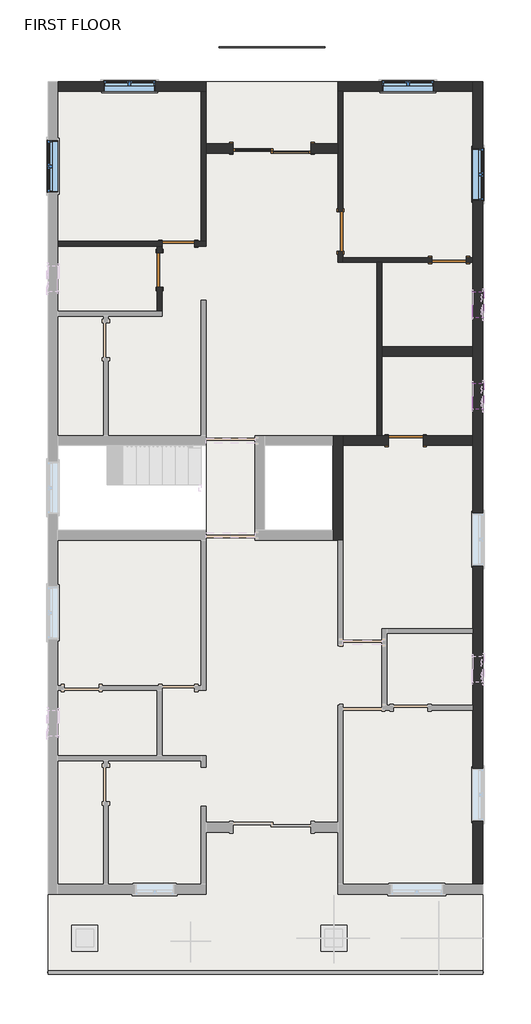
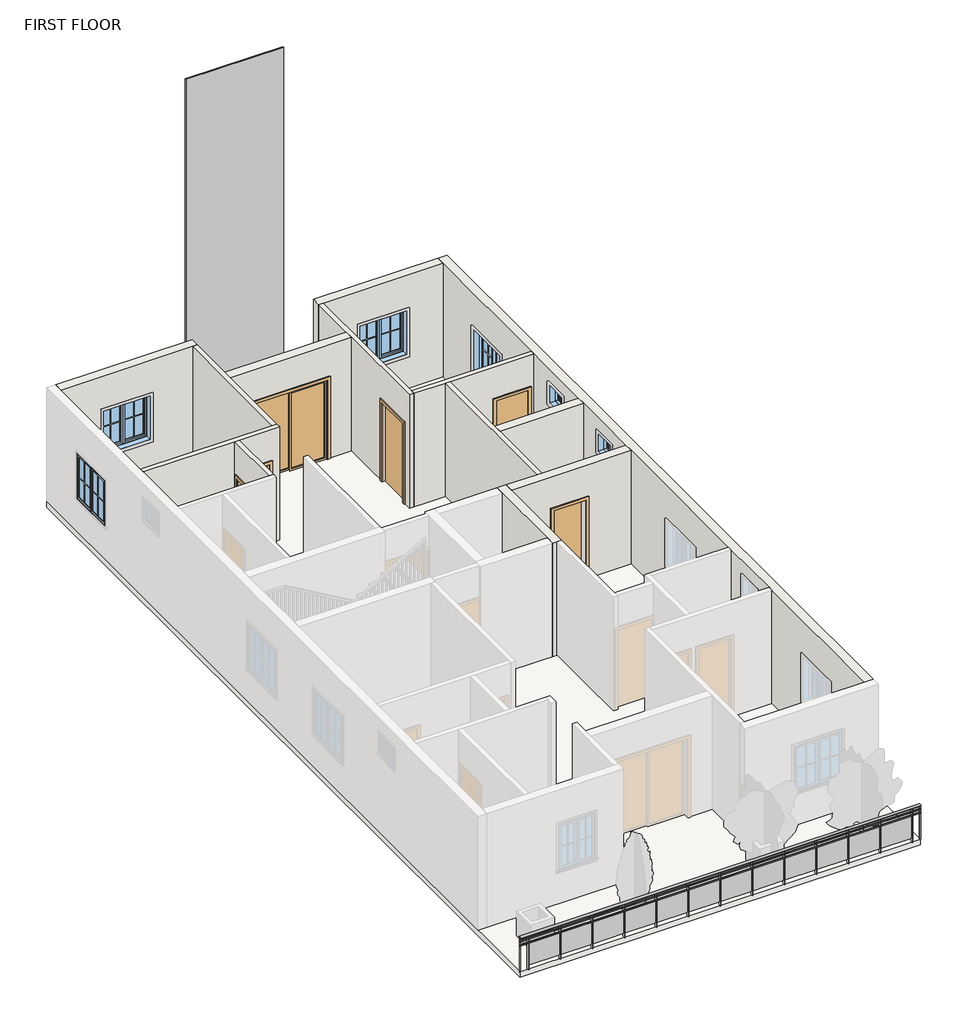
# One storey, part 2 of 4: 13 walls, 6 doors, 6 windows, 1 plate, 1 railing, 1 slab.
"""IFC4 building model written with IfcOpenShell, lengths in millimetres."""

from ifc_helpers import new_model, si_unit, point, frame, origin, place, context, project, spatial, polyline, ellipse_curve, trimmed, outline, extrude, faceted_brep, transform, mapped, element, save
from ifc_brep_helpers import plane_surface, extruded_surface, advanced_brep
from components import door_d4d75d1e, door_214872d5, door_d141acb4, door_38851409, door_7b345704, single_flush_3_x7_e5f9f3c4, system_panel_glazed_b4ce2d81, window_79894727, window_casement_double_4_x4_af3140d2

model = new_model("IFC4")

# Units and contexts
model_context = context("Model", 3, world=origin())
ifc_project = project(units=[si_unit("LENGTHUNIT", "METRE", prefix="MILLI")], contexts=[model_context])

# Site, building, storey
site = spatial("IfcSite", under=ifc_project)
building = spatial("IfcBuilding", under=site)
storey = spatial("IfcBuildingStorey", under=building, Name="FIRST FLOOR", Elevation=3200.4)

# Doors
placement = place(None, origin())
door_shape = door_d4d75d1e(model_context)
element("IfcDoor", 1, ObjectType="Door-Double-Sliding : 72\" x 84\"", at=placement, inside=storey, context=model_context, shape_type="MappedRepresentation", body=[
    mapped(door_shape, transform((-1119.4789041, 8623.7153263, 3200.4), x_axis=(-1.0, 0.0, 0.0), y_axis=(0.0, -1.0, 0.0), z_axis=(0.0, 0.0, 1.0))),
])
door_2_shape = door_214872d5(model_context)
element("IfcDoor", 2, ObjectType="Single-Flush : 2'6\"X7'", at=placement, inside=storey, context=model_context, shape_type="MappedRepresentation", body=[
    mapped(door_2_shape, transform((-3310.2289041, 6267.8653263, 3200.4), x_axis=(1.0, 0.0, 0.0), y_axis=(0.0, 1.0, 0.0), z_axis=(0.0, 0.0, 1.0))),
])
door_3_shape = door_d141acb4(model_context)
element("IfcDoor", 3, ObjectType="Single-Flush : 2'8\"X7'", at=placement, inside=storey, context=model_context, shape_type="MappedRepresentation", body=[
    mapped(door_3_shape, transform((-3748.3789041, 5651.9153263, 3200.4), x_axis=(0.0, 1.0, 0.0), y_axis=(-1.0, 0.0, 0.0), z_axis=(0.0, 0.0, 1.0))),
])
door_4_shape = door_38851409(model_context)
element("IfcDoor", 4, ObjectType="Single-Flush : 2'8\"X7'", at=placement, inside=storey, context=model_context, shape_type="MappedRepresentation", body=[
    mapped(door_4_shape, transform((3027.0710959, 5886.8653263, 3200.4), x_axis=(1.0, 0.0, 0.0), y_axis=(0.0, 1.0, 0.0), z_axis=(0.0, 0.0, 1.0))),
])
door_5_shape = door_7b345704(model_context)
element("IfcDoor", 5, ObjectType="Single-Flush : 2'8\"X7'", at=placement, inside=storey, context=model_context, shape_type="MappedRepresentation", body=[
    mapped(door_5_shape, transform((2011.0710959, 1664.1153263, 3200.4), x_axis=(-1.0, 0.0, 0.0), y_axis=(0.0, -1.0, 0.0), z_axis=(0.0, 0.0, 1.0))),
])
single_flush_3_x7_shape = single_flush_3_x7_e5f9f3c4(model_context)
element("IfcDoor", 6, ObjectType="Single-Flush : 3'X7'", at=placement, inside=storey, context=model_context, shape_type="MappedRepresentation", body=[
    mapped(single_flush_3_x7_shape, transform((480.7210959, 6553.6153263, 3200.4), x_axis=(0.0, -1.0, 0.0), y_axis=(1.0, 0.0, 0.0), z_axis=(0.0, 0.0, 1.0))),
])

# Plate
system_panel_glazed_shape = system_panel_glazed_b4ce2d81(model_context)
element("IfcPlate", 7, ObjectType="System Panel : Glazed", at=placement, inside=storey, context=model_context, shape_type="MappedRepresentation", body=[
    mapped(system_panel_glazed_shape, transform((-1119.4789041, 10833.5153263, 3200.4), x_axis=(1.0, 0.0, 0.0), y_axis=(0.0, 1.0, 0.0), z_axis=(0.0, 0.0, 1.0))),
])

# Railing
element("IfcRailing", 8, ObjectType="Glass Panel - Bottom Fill", at=placement, inside=storey, context=model_context, shape_type="SolidModel", body=[
    advanced_brep(
    [(-6358.2289041, -10731.0846737, 4114.8), (-6358.2289041, -10807.2846737, 4114.8), (3814.4710959, -10731.0846737, 4114.8), (3814.4710959, -10807.2846737, 4114.8)],
    [
        (0, 1, ellipse_curve(frame((-6358.2289041, -10769.1846737, 4114.8), z_axis=(-1.0, 0.0, 0.0), x_axis=(0.0, -1.0, 0.0)), 38.1, 28.575)),
        (1, 0, ellipse_curve(frame((-6358.2289041, -10769.1846737, 4114.8), z_axis=(-1.0, 0.0, 0.0), x_axis=(0.0, -1.0, 0.0)), 38.1, 28.575)),
        (2, 3, ellipse_curve(frame((3814.4710959, -10769.1846737, 4114.8), z_axis=(1.0, 0.0, 0.0), x_axis=(0.0, -1.0, 0.0)), 38.1, 28.575)),
        (3, 2, ellipse_curve(frame((3814.4710959, -10769.1846737, 4114.8), z_axis=(1.0, 0.0, 0.0), x_axis=(0.0, -1.0, 0.0)), 38.1, 28.575)),
        (0, 2),
        (3, 1),
    ],
    [
        plane_surface(frame((-6358.2289041, -10769.1846737, 4114.8), z_axis=(-1.0, 0.0, 0.0), x_axis=(0.0, 1.0, 0.0))),
        plane_surface(frame((3814.4710959, -10769.1846737, 4114.8), z_axis=(1.0, 0.0, 0.0), x_axis=(0.0, 1.0, 0.0))),
        extruded_surface(trimmed(ellipse_curve(frame((3814.4710959, -10769.1846737, 4114.8), z_axis=(-1.0, 0.0, 0.0), x_axis=(0.0, -1.0, 0.0)), 38.1, 28.575), [point((3814.4710959, -10731.0846737, 4114.8))], [point((3814.4710959, -10807.2846737, 4114.8))], True, "CARTESIAN"), (-10172.7, 0.0, 0.0), 10172.7),
        extruded_surface(trimmed(ellipse_curve(frame((3814.4710959, -10769.1846737, 4114.8), z_axis=(-1.0, 0.0, 0.0), x_axis=(0.0, -1.0, 0.0)), 38.1, 28.575), [point((3814.4710959, -10807.2846737, 4114.8))], [point((3814.4710959, -10731.0846737, 4114.8))], True, "CARTESIAN"), (-10172.7, 0.0, 0.0), 10172.7),
    ],
    [
        (0, [[1, 2]]),
        (1, [[3, 4]]),
        (2, [[-1, 5, -4, 6]]),
        (3, [[-2, -6, -3, -5]]),
    ],
),
    extrude(outline(polyline([(-6358.2289041, -10781.8846737), (-6358.2289041, -10756.4846737), (3814.4710959, -10756.4846737), (3814.4710959, -10781.8846737), (-6358.2289041, -10781.8846737)])), frame((0.0, 0.0, 4000.5), z_axis=(0.0, 0.0, 1.0), x_axis=(1.0, 0.0, 0.0)), (0.0, 0.0, 1.0), 25.4),
    extrude(outline(polyline([(-6358.2289041, -10781.8846737), (-6358.2289041, -10756.4846737), (3814.4710959, -10756.4846737), (3814.4710959, -10781.8846737), (-6358.2289041, -10781.8846737)])), frame((0.0, 0.0, 3898.9), z_axis=(0.0, 0.0, 1.0), x_axis=(1.0, 0.0, 0.0)), (0.0, 0.0, 1.0), 25.4),
    extrude(outline(polyline([(3598.5710959, -10794.5846737), (3598.5710959, -10743.7846737), (3611.2710959, -10743.7846737), (3611.2710959, -10794.5846737), (3598.5710959, -10794.5846737)])), frame((0.0, 0.0, 3200.4), z_axis=(0.0, 0.0, 1.0), x_axis=(1.0, 0.0, 0.0)), (0.0, 0.0, 1.0), 885.825),
    extrude(outline(polyline([(2792.1210959, -10762.6495167), (3604.9210959, -10762.6495167), (3604.9210959, -10768.9995167), (2792.1210959, -10768.9995167), (2792.1210959, -10762.6495167)])), frame((0.0, 0.0, 3302.0), z_axis=(0.0, 0.0, 1.0), x_axis=(1.0, 0.0, 0.0)), (0.0, 0.0, 1.0), 596.9),
    extrude(outline(polyline([(2785.7710959, -10794.5846737), (2785.7710959, -10743.7846737), (2798.4710959, -10743.7846737), (2798.4710959, -10794.5846737), (2785.7710959, -10794.5846737)])), frame((0.0, 0.0, 3200.4), z_axis=(0.0, 0.0, 1.0), x_axis=(1.0, 0.0, 0.0)), (0.0, 0.0, 1.0), 885.825),
    extrude(outline(polyline([(1979.3210959, -10762.6495167), (2792.1210959, -10762.6495167), (2792.1210959, -10768.9995167), (1979.3210959, -10768.9995167), (1979.3210959, -10762.6495167)])), frame((0.0, 0.0, 3302.0), z_axis=(0.0, 0.0, 1.0), x_axis=(1.0, 0.0, 0.0)), (0.0, 0.0, 1.0), 596.9),
    extrude(outline(polyline([(1972.9710959, -10794.5846737), (1972.9710959, -10743.7846737), (1985.6710959, -10743.7846737), (1985.6710959, -10794.5846737), (1972.9710959, -10794.5846737)])), frame((0.0, 0.0, 3200.4), z_axis=(0.0, 0.0, 1.0), x_axis=(1.0, 0.0, 0.0)), (0.0, 0.0, 1.0), 885.825),
    extrude(outline(polyline([(1166.5210959, -10762.6495167), (1979.3210959, -10762.6495167), (1979.3210959, -10768.9995167), (1166.5210959, -10768.9995167), (1166.5210959, -10762.6495167)])), frame((0.0, 0.0, 3302.0), z_axis=(0.0, 0.0, 1.0), x_axis=(1.0, 0.0, 0.0)), (0.0, 0.0, 1.0), 596.9),
    extrude(outline(polyline([(1160.1710959, -10794.5846737), (1160.1710959, -10743.7846737), (1172.8710959, -10743.7846737), (1172.8710959, -10794.5846737), (1160.1710959, -10794.5846737)])), frame((0.0, 0.0, 3200.4), z_axis=(0.0, 0.0, 1.0), x_axis=(1.0, 0.0, 0.0)), (0.0, 0.0, 1.0), 885.825),
    extrude(outline(polyline([(353.7210959, -10762.6495167), (1166.5210959, -10762.6495167), (1166.5210959, -10768.9995167), (353.7210959, -10768.9995167), (353.7210959, -10762.6495167)])), frame((0.0, 0.0, 3302.0), z_axis=(0.0, 0.0, 1.0), x_axis=(1.0, 0.0, 0.0)), (0.0, 0.0, 1.0), 596.9),
    extrude(outline(polyline([(347.3710959, -10794.5846737), (347.3710959, -10743.7846737), (360.0710959, -10743.7846737), (360.0710959, -10794.5846737), (347.3710959, -10794.5846737)])), frame((0.0, 0.0, 3200.4), z_axis=(0.0, 0.0, 1.0), x_axis=(1.0, 0.0, 0.0)), (0.0, 0.0, 1.0), 885.825),
    extrude(outline(polyline([(-459.0789041, -10762.6495167), (353.7210959, -10762.6495167), (353.7210959, -10768.9995167), (-459.0789041, -10768.9995167), (-459.0789041, -10762.6495167)])), frame((0.0, 0.0, 3302.0), z_axis=(0.0, 0.0, 1.0), x_axis=(1.0, 0.0, 0.0)), (0.0, 0.0, 1.0), 596.9),
    extrude(outline(polyline([(-465.4289041, -10794.5846737), (-465.4289041, -10743.7846737), (-452.7289041, -10743.7846737), (-452.7289041, -10794.5846737), (-465.4289041, -10794.5846737)])), frame((0.0, 0.0, 3200.4), z_axis=(0.0, 0.0, 1.0), x_axis=(1.0, 0.0, 0.0)), (0.0, 0.0, 1.0), 885.825),
    extrude(outline(polyline([(-1271.8789041, -10762.6495167), (-459.0789041, -10762.6495167), (-459.0789041, -10768.9995167), (-1271.8789041, -10768.9995167), (-1271.8789041, -10762.6495167)])), frame((0.0, 0.0, 3302.0), z_axis=(0.0, 0.0, 1.0), x_axis=(1.0, 0.0, 0.0)), (0.0, 0.0, 1.0), 596.9),
    extrude(outline(polyline([(-1278.2289041, -10794.5846737), (-1278.2289041, -10743.7846737), (-1265.5289041, -10743.7846737), (-1265.5289041, -10794.5846737), (-1278.2289041, -10794.5846737)])), frame((0.0, 0.0, 3200.4), z_axis=(0.0, 0.0, 1.0), x_axis=(1.0, 0.0, 0.0)), (0.0, 0.0, 1.0), 885.825),
    extrude(outline(polyline([(-2084.6789041, -10762.6495167), (-1271.8789041, -10762.6495167), (-1271.8789041, -10768.9995167), (-2084.6789041, -10768.9995167), (-2084.6789041, -10762.6495167)])), frame((0.0, 0.0, 3302.0), z_axis=(0.0, 0.0, 1.0), x_axis=(1.0, 0.0, 0.0)), (0.0, 0.0, 1.0), 596.9),
    extrude(outline(polyline([(-2091.0289041, -10794.5846737), (-2091.0289041, -10743.7846737), (-2078.3289041, -10743.7846737), (-2078.3289041, -10794.5846737), (-2091.0289041, -10794.5846737)])), frame((0.0, 0.0, 3200.4), z_axis=(0.0, 0.0, 1.0), x_axis=(1.0, 0.0, 0.0)), (0.0, 0.0, 1.0), 885.825),
    extrude(outline(polyline([(-2897.4789041, -10762.6495167), (-2084.6789041, -10762.6495167), (-2084.6789041, -10768.9995167), (-2897.4789041, -10768.9995167), (-2897.4789041, -10762.6495167)])), frame((0.0, 0.0, 3302.0), z_axis=(0.0, 0.0, 1.0), x_axis=(1.0, 0.0, 0.0)), (0.0, 0.0, 1.0), 596.9),
    extrude(outline(polyline([(-2903.8289041, -10794.5846737), (-2903.8289041, -10743.7846737), (-2891.1289041, -10743.7846737), (-2891.1289041, -10794.5846737), (-2903.8289041, -10794.5846737)])), frame((0.0, 0.0, 3200.4), z_axis=(0.0, 0.0, 1.0), x_axis=(1.0, 0.0, 0.0)), (0.0, 0.0, 1.0), 885.825),
    extrude(outline(polyline([(-3710.2789041, -10762.6495167), (-2897.4789041, -10762.6495167), (-2897.4789041, -10768.9995167), (-3710.2789041, -10768.9995167), (-3710.2789041, -10762.6495167)])), frame((0.0, 0.0, 3302.0), z_axis=(0.0, 0.0, 1.0), x_axis=(1.0, 0.0, 0.0)), (0.0, 0.0, 1.0), 596.9),
    extrude(outline(polyline([(-3716.6289041, -10794.5846737), (-3716.6289041, -10743.7846737), (-3703.9289041, -10743.7846737), (-3703.9289041, -10794.5846737), (-3716.6289041, -10794.5846737)])), frame((0.0, 0.0, 3200.4), z_axis=(0.0, 0.0, 1.0), x_axis=(1.0, 0.0, 0.0)), (0.0, 0.0, 1.0), 885.825),
    extrude(outline(polyline([(-4523.0789041, -10762.6495167), (-3710.2789041, -10762.6495167), (-3710.2789041, -10768.9995167), (-4523.0789041, -10768.9995167), (-4523.0789041, -10762.6495167)])), frame((0.0, 0.0, 3302.0), z_axis=(0.0, 0.0, 1.0), x_axis=(1.0, 0.0, 0.0)), (0.0, 0.0, 1.0), 596.9),
    extrude(outline(polyline([(-4529.4289041, -10794.5846737), (-4529.4289041, -10743.7846737), (-4516.7289041, -10743.7846737), (-4516.7289041, -10794.5846737), (-4529.4289041, -10794.5846737)])), frame((0.0, 0.0, 3200.4), z_axis=(0.0, 0.0, 1.0), x_axis=(1.0, 0.0, 0.0)), (0.0, 0.0, 1.0), 885.825),
    extrude(outline(polyline([(-5335.8789041, -10762.6495167), (-4523.0789041, -10762.6495167), (-4523.0789041, -10768.9995167), (-5335.8789041, -10768.9995167), (-5335.8789041, -10762.6495167)])), frame((0.0, 0.0, 3302.0), z_axis=(0.0, 0.0, 1.0), x_axis=(1.0, 0.0, 0.0)), (0.0, 0.0, 1.0), 596.9),
    extrude(outline(polyline([(-5342.2289041, -10794.5846737), (-5342.2289041, -10743.7846737), (-5329.5289041, -10743.7846737), (-5329.5289041, -10794.5846737), (-5342.2289041, -10794.5846737)])), frame((0.0, 0.0, 3200.4), z_axis=(0.0, 0.0, 1.0), x_axis=(1.0, 0.0, 0.0)), (0.0, 0.0, 1.0), 885.825),
    extrude(outline(polyline([(-6148.6789041, -10762.6495167), (-5335.8789041, -10762.6495167), (-5335.8789041, -10768.9995167), (-6148.6789041, -10768.9995167), (-6148.6789041, -10762.6495167)])), frame((0.0, 0.0, 3302.0), z_axis=(0.0, 0.0, 1.0), x_axis=(1.0, 0.0, 0.0)), (0.0, 0.0, 1.0), 596.9),
    extrude(outline(polyline([(-6155.0289041, -10794.5846737), (-6155.0289041, -10743.7846737), (-6142.3289041, -10743.7846737), (-6142.3289041, -10794.5846737), (-6155.0289041, -10794.5846737)])), frame((0.0, 0.0, 3200.4), z_axis=(0.0, 0.0, 1.0), x_axis=(1.0, 0.0, 0.0)), (0.0, 0.0, 1.0), 885.825),
    extrude(outline(polyline([(3801.7710959, -10778.7096737), (3801.7710959, -10759.6596737), (3820.8210959, -10759.6596737), (3820.8210959, -10778.7096737), (3801.7710959, -10778.7096737)])), frame((0.0, 0.0, 3200.4), z_axis=(0.0, 0.0, 1.0), x_axis=(1.0, 0.0, 0.0)), (0.0, 0.0, 1.0), 885.825),
    extrude(outline(polyline([(-6364.5789041, -10778.7096737), (-6364.5789041, -10759.6596737), (-6345.5289041, -10759.6596737), (-6345.5289041, -10778.7096737), (-6364.5789041, -10778.7096737)])), frame((0.0, 0.0, 3200.4), z_axis=(0.0, 0.0, 1.0), x_axis=(1.0, 0.0, 0.0)), (0.0, 0.0, 1.0), 885.825),
])

# Slab
element("IfcSlab", 9, ObjectType="6\"", at=placement, inside=storey, context=model_context, shape_type="SweptSolid", body=[
    extrude(outline(polyline([(3814.4710959, 10058.8153263), (3814.4710959, -10769.1846737), (-6358.2289041, -10769.1846737), (-6358.2289041, 10058.8153263), (3814.4710959, 10058.8153263)]), holes=[polyline([(-2662.5289041, 1549.8153263), (-6129.6289041, 1549.8153263), (-6129.6289041, -431.3846737), (-2662.5289041, -431.3846737), (-2662.5289041, 1549.8153263)]), polyline([(537.8710959, 1778.4153263), (-1519.5289041, 1778.4153263), (-1519.5289041, -659.9846737), (537.8710959, -659.9846737), (537.8710959, 1778.4153263)])]), frame((0.0, 0.0, 3048.0), z_axis=(0.0, 0.0, 1.0), x_axis=(1.0, 0.0, 0.0)), (0.0, 0.0, 1.0), 152.4),
])

# Walls
element("IfcWall", 10, ObjectType="4.5\"", at=placement, inside=storey, context=model_context, shape_type="SweptSolid", body=[
    extrude(outline(polyline([(6210.7153263, 3200.4), (6058.3153263, 3200.4), (6058.3153263, 5334.0), (5245.5153263, 5334.0), (5245.5153263, 3200.4), (4686.7153263, 3200.4), (4686.7153263, 6248.4), (6210.7153263, 6248.4), (6210.7153263, 3200.4)])), frame((-3805.5289041, 0.0, 0.0), z_axis=(1.0, 0.0, 0.0), x_axis=(0.0, 1.0, 0.0)), (0.0, 0.0, 1.0), 114.3),
])
element("IfcWall", 11, ObjectType="4.5\"", at=placement, inside=storey, context=model_context, shape_type="Brep", body=[
    faceted_brep([(-2929.2289041, 6210.7153263, 5334.0), (-2929.2289041, 6210.7153263, 3200.4), (-2662.5289041, 6210.7153263, 3200.4), (-2662.5289041, 6210.7153263, 6248.4), (-3691.2289041, 6210.7153263, 6248.4), (-3805.5289041, 6210.7153263, 6248.4), (-6129.6289041, 6210.7153263, 6248.4), (-6129.6289041, 6210.7153263, 3200.4), (-3805.5289041, 6210.7153263, 3200.4), (-3691.2289041, 6210.7153263, 3200.4), (-3691.2289041, 6210.7153263, 5334.0), (-2662.5289041, 6325.0153263, 3200.4), (-2776.8289041, 6325.0153263, 3200.4), (-2929.2289041, 6325.0153263, 3200.4), (-2929.2289041, 6325.0153263, 5334.0), (-3691.2289041, 6325.0153263, 5334.0), (-3691.2289041, 6325.0153263, 3200.4), (-6129.6289041, 6325.0153263, 3200.4), (-6129.6289041, 6325.0153263, 6248.4), (-2776.8289041, 6325.0153263, 6248.4), (-2662.5289041, 6325.0153263, 6248.4)], [[[0, 1, 2, 3, 4, 5, 6, 7, 8, 9, 10]], [[11, 12, 13, 14, 15, 16, 17, 18, 19, 20]], [[2, 1, 13, 12, 11]], [[9, 8, 7, 17, 16]], [[6, 5, 4, 3, 20, 19, 18]], [[7, 6, 18, 17]], [[3, 2, 11, 20]], [[14, 13, 1, 0]], [[15, 14, 0, 10]], [[16, 15, 10, 9]]]),
])
element("IfcWall", 12, ObjectType="4.5\"", at=placement, inside=storey, context=model_context, shape_type="Brep", body=[
    faceted_brep([(-2662.5289041, 6325.0153263, 3200.4), (-2662.5289041, 8382.4153263, 3200.4), (-2662.5289041, 8611.0153263, 3200.4), (-2662.5289041, 9830.2153263, 3200.4), (-2662.5289041, 9830.2153263, 6248.4), (-2662.5289041, 8611.0153263, 6248.4), (-2662.5289041, 8382.4153263, 6248.4), (-2662.5289041, 6325.0153263, 6248.4), (-2776.8289041, 6325.0153263, 3200.4), (-2776.8289041, 6325.0153263, 6248.4), (-2776.8289041, 9830.2153263, 6248.4), (-2776.8289041, 9830.2153263, 3200.4)], [[[0, 1, 2, 3, 4, 5, 6, 7]], [[8, 9, 10, 11]], [[3, 2, 1, 0, 8, 11]], [[7, 6, 5, 4, 10, 9]], [[0, 7, 9, 8]], [[4, 3, 11, 10]]]),
])
element("IfcWall", 13, ObjectType="4.5\"", at=placement, inside=storey, context=model_context, shape_type="Brep", body=[
    faceted_brep([(423.5710959, 6096.4153263, 5334.0), (423.5710959, 6096.4153263, 3200.4), (423.5710959, 5829.7153263, 3200.4), (423.5710959, 5829.7153263, 6248.4), (423.5710959, 8382.4153263, 6248.4), (423.5710959, 8611.0153263, 6248.4), (423.5710959, 9830.2153263, 6248.4), (423.5710959, 9830.2153263, 3200.4), (423.5710959, 8611.0153263, 3200.4), (423.5710959, 8382.4153263, 3200.4), (423.5710959, 7010.8153263, 3200.4), (423.5710959, 7010.8153263, 5334.0), (537.8710959, 5829.7153263, 3200.4), (537.8710959, 5944.0153263, 3200.4), (537.8710959, 6096.4153263, 3200.4), (537.8710959, 6096.4153263, 5334.0), (537.8710959, 7010.8153263, 5334.0), (537.8710959, 7010.8153263, 3200.4), (537.8710959, 9830.2153263, 3200.4), (537.8710959, 9830.2153263, 6248.4), (537.8710959, 5944.0153263, 6248.4), (537.8710959, 5829.7153263, 6248.4)], [[[0, 1, 2, 3, 4, 5, 6, 7, 8, 9, 10, 11]], [[12, 13, 14, 15, 16, 17, 18, 19, 20, 21]], [[2, 1, 14, 13, 12]], [[10, 9, 8, 7, 18, 17]], [[6, 5, 4, 3, 21, 20, 19]], [[7, 6, 19, 18]], [[3, 2, 12, 21]], [[15, 14, 1, 0]], [[16, 15, 0, 11]], [[17, 16, 11, 10]]]),
])
element("IfcWall", 14, ObjectType="4.5\"", at=placement, inside=storey, context=model_context, shape_type="Brep", body=[
    faceted_brep([(3433.4710959, 5829.7153263, 5334.0), (3433.4710959, 5829.7153263, 3200.4), (3585.8710959, 5829.7153263, 3200.4), (3585.8710959, 5829.7153263, 6248.4), (1452.2710959, 5829.7153263, 6248.4), (1337.9710959, 5829.7153263, 6248.4), (537.8710959, 5829.7153263, 6248.4), (537.8710959, 5829.7153263, 3200.4), (1337.9710959, 5829.7153263, 3200.4), (1452.2710959, 5829.7153263, 3200.4), (2620.6710959, 5829.7153263, 3200.4), (2620.6710959, 5829.7153263, 5334.0), (3585.8710959, 5944.0153263, 3200.4), (3433.4710959, 5944.0153263, 3200.4), (3433.4710959, 5944.0153263, 5334.0), (2620.6710959, 5944.0153263, 5334.0), (2620.6710959, 5944.0153263, 3200.4), (537.8710959, 5944.0153263, 3200.4), (537.8710959, 5944.0153263, 6248.4), (3585.8710959, 5944.0153263, 6248.4)], [[[0, 1, 2, 3, 4, 5, 6, 7, 8, 9, 10, 11]], [[12, 13, 14, 15, 16, 17, 18, 19]], [[2, 1, 13, 12]], [[10, 9, 8, 7, 17, 16]], [[6, 5, 4, 3, 19, 18]], [[7, 6, 18, 17]], [[3, 2, 12, 19]], [[14, 13, 1, 0]], [[15, 14, 0, 11]], [[16, 15, 11, 10]]]),
])
element("IfcWall", 15, ObjectType="4.5\"", at=placement, inside=storey, context=model_context, shape_type="Brep", body=[
    faceted_brep([(1337.9710959, 5829.7153263, 3200.4), (1337.9710959, 1778.4153263, 3200.4), (1337.9710959, 1778.4153263, 6248.4), (1337.9710959, 5829.7153263, 6248.4), (1452.2710959, 5829.7153263, 3200.4), (1452.2710959, 5829.7153263, 6248.4), (1452.2710959, 3861.2153263, 6248.4), (1452.2710959, 3632.6153263, 6248.4), (1452.2710959, 1778.4153263, 6248.4), (1452.2710959, 1778.4153263, 3200.4), (1452.2710959, 3632.6153263, 3200.4), (1452.2710959, 3861.2153263, 3200.4)], [[[0, 1, 2, 3]], [[4, 5, 6, 7, 8, 9, 10, 11]], [[1, 0, 4, 11, 10, 9]], [[3, 2, 8, 7, 6, 5]], [[2, 1, 9, 8]], [[0, 3, 5, 4]]]),
])
element("IfcWall", 16, ObjectType="9\"", at=placement, inside=storey, context=model_context, shape_type="Brep", body=[
    faceted_brep([(3814.4710959, -8711.7846737, 3200.4), (3814.4710959, 10058.8153263, 3200.4), (3814.4710959, 10058.8153263, 6248.4), (3814.4710959, -8711.7846737, 6248.4), (3814.4710959, -7225.8846737, 5334.0), (3814.4710959, -6006.6846737, 5334.0), (3814.4710959, -6006.6846737, 4114.8), (3814.4710959, -7225.8846737, 4114.8), (3814.4710959, -1256.8846737, 5334.0), (3814.4710959, -37.6846737, 5334.0), (3814.4710959, -37.6846737, 4114.8), (3814.4710959, -1256.8846737, 4114.8), (3814.4710959, 7277.5153263, 5334.0), (3814.4710959, 8496.7153263, 5334.0), (3814.4710959, 8496.7153263, 4114.8), (3814.4710959, 7277.5153263, 4114.8), (3814.4710959, -3987.3846737, 5867.4), (3814.4710959, -3377.7846737, 5867.4), (3814.4710959, -3377.7846737, 5334.0), (3814.4710959, -3987.3846737, 5334.0), (3814.4710959, 2400.7153263, 5867.4), (3814.4710959, 3010.3153263, 5867.4), (3814.4710959, 3010.3153263, 5334.0), (3814.4710959, 2400.7153263, 5334.0), (3814.4710959, 4540.6653263, 5867.4), (3814.4710959, 5150.2653263, 5867.4), (3814.4710959, 5150.2653263, 5334.0), (3814.4710959, 4540.6653263, 5334.0), (3585.8710959, -8711.7846737, 3200.4), (3585.8710959, -8711.7846737, 6248.4), (3585.8710959, -4635.0846737, 6248.4), (3585.8710959, -4520.7846737, 6248.4), (3585.8710959, -2844.3846737, 6248.4), (3585.8710959, -2730.0846737, 6248.4), (3585.8710959, 1549.8153263, 6248.4), (3585.8710959, 1778.4153263, 6248.4), (3585.8710959, 3632.6153263, 6248.4), (3585.8710959, 3861.2153263, 6248.4), (3585.8710959, 5829.7153263, 6248.4), (3585.8710959, 5944.0153263, 6248.4), (3585.8710959, 9830.2153263, 6248.4), (3585.8710959, 10058.8153263, 6248.4), (3585.8710959, 10058.8153263, 3200.4), (3585.8710959, 9830.2153263, 3200.4), (3585.8710959, 5944.0153263, 3200.4), (3585.8710959, 5829.7153263, 3200.4), (3585.8710959, 3861.2153263, 3200.4), (3585.8710959, 3632.6153263, 3200.4), (3585.8710959, 1778.4153263, 3200.4), (3585.8710959, 1549.8153263, 3200.4), (3585.8710959, -2730.0846737, 3200.4), (3585.8710959, -2844.3846737, 3200.4), (3585.8710959, -4520.7846737, 3200.4), (3585.8710959, -4635.0846737, 3200.4), (3585.8710959, -7225.8846737, 5334.0), (3585.8710959, -7225.8846737, 4114.8), (3585.8710959, -6006.6846737, 4114.8), (3585.8710959, -6006.6846737, 5334.0), (3585.8710959, -1256.8846737, 5334.0), (3585.8710959, -1256.8846737, 4114.8), (3585.8710959, -37.6846737, 4114.8), (3585.8710959, -37.6846737, 5334.0), (3585.8710959, 7277.5153263, 5334.0), (3585.8710959, 7277.5153263, 4114.8), (3585.8710959, 8496.7153263, 4114.8), (3585.8710959, 8496.7153263, 5334.0), (3585.8710959, -3987.3846737, 5867.4), (3585.8710959, -3987.3846737, 5334.0), (3585.8710959, -3377.7846737, 5334.0), (3585.8710959, -3377.7846737, 5867.4), (3585.8710959, 2400.7153263, 5867.4), (3585.8710959, 2400.7153263, 5334.0), (3585.8710959, 3010.3153263, 5334.0), (3585.8710959, 3010.3153263, 5867.4), (3585.8710959, 4540.6653263, 5867.4), (3585.8710959, 4540.6653263, 5334.0), (3585.8710959, 5150.2653263, 5334.0), (3585.8710959, 5150.2653263, 5867.4)], [[[0, 1, 2, 3], [4, 5, 6, 7], [8, 9, 10, 11], [12, 13, 14, 15], [16, 17, 18, 19], [20, 21, 22, 23], [24, 25, 26, 27]], [[28, 29, 30, 31, 32, 33, 34, 35, 36, 37, 38, 39, 40, 41, 42, 43, 44, 45, 46, 47, 48, 49, 50, 51, 52, 53], [54, 55, 56, 57], [58, 59, 60, 61], [62, 63, 64, 65], [66, 67, 68, 69], [70, 71, 72, 73], [74, 75, 76, 77]], [[1, 0, 28, 53, 52, 51, 50, 49, 48, 47, 46, 45, 44, 43, 42]], [[3, 2, 41, 40, 39, 38, 37, 36, 35, 34, 33, 32, 31, 30, 29]], [[0, 3, 29, 28]], [[2, 1, 42, 41]], [[55, 54, 4, 7]], [[56, 55, 7, 6]], [[57, 56, 6, 5]], [[54, 57, 5, 4]], [[59, 58, 8, 11]], [[60, 59, 11, 10]], [[61, 60, 10, 9]], [[58, 61, 9, 8]], [[63, 62, 12, 15]], [[64, 63, 15, 14]], [[65, 64, 14, 13]], [[62, 65, 13, 12]], [[67, 66, 16, 19]], [[68, 67, 19, 18]], [[69, 68, 18, 17]], [[66, 69, 17, 16]], [[71, 70, 20, 23]], [[72, 71, 23, 22]], [[73, 72, 22, 21]], [[70, 73, 21, 20]], [[75, 74, 24, 27]], [[76, 75, 27, 26]], [[77, 76, 26, 25]], [[74, 77, 25, 24]]]),
])
element("IfcWall", 17, ObjectType="9\"", at=placement, inside=storey, context=model_context, shape_type="Brep", body=[
    faceted_brep([(3585.8710959, 10058.8153263, 3200.4), (423.5710959, 10058.8153263, 3200.4), (423.5710959, 10058.8153263, 6248.4), (3585.8710959, 10058.8153263, 6248.4), (2671.4710959, 10058.8153263, 5334.0), (1452.2710959, 10058.8153263, 5334.0), (1452.2710959, 10058.8153263, 4114.8), (2671.4710959, 10058.8153263, 4114.8), (3585.8710959, 9830.2153263, 3200.4), (3585.8710959, 9830.2153263, 6248.4), (537.8710959, 9830.2153263, 6248.4), (423.5710959, 9830.2153263, 6248.4), (423.5710959, 9830.2153263, 3200.4), (537.8710959, 9830.2153263, 3200.4), (2671.4710959, 9830.2153263, 5334.0), (2671.4710959, 9830.2153263, 4114.8), (1452.2710959, 9830.2153263, 4114.8), (1452.2710959, 9830.2153263, 5334.0)], [[[0, 1, 2, 3], [4, 5, 6, 7]], [[8, 9, 10, 11, 12, 13], [14, 15, 16, 17]], [[1, 0, 8, 13, 12]], [[3, 2, 11, 10, 9]], [[0, 3, 9, 8]], [[2, 1, 12, 11]], [[15, 14, 4, 7]], [[16, 15, 7, 6]], [[17, 16, 6, 5]], [[14, 17, 5, 4]]]),
])
element("IfcWall", 18, ObjectType="9\"", at=placement, inside=storey, context=model_context, shape_type="Brep", body=[
    faceted_brep([(-2662.5289041, 10058.8153263, 3200.4), (-6129.6289041, 10058.8153263, 3200.4), (-6129.6289041, 10058.8153263, 6248.4), (-2662.5289041, 10058.8153263, 6248.4), (-3843.6289041, 10058.8153263, 5334.0), (-5062.8289041, 10058.8153263, 5334.0), (-5062.8289041, 10058.8153263, 4114.8), (-3843.6289041, 10058.8153263, 4114.8), (-2662.5289041, 9830.2153263, 3200.4), (-2662.5289041, 9830.2153263, 6248.4), (-2776.8289041, 9830.2153263, 6248.4), (-6129.6289041, 9830.2153263, 6248.4), (-6129.6289041, 9830.2153263, 3200.4), (-2776.8289041, 9830.2153263, 3200.4), (-3843.6289041, 9830.2153263, 5334.0), (-3843.6289041, 9830.2153263, 4114.8), (-5062.8289041, 9830.2153263, 4114.8), (-5062.8289041, 9830.2153263, 5334.0)], [[[0, 1, 2, 3], [4, 5, 6, 7]], [[8, 9, 10, 11, 12, 13], [14, 15, 16, 17]], [[1, 0, 8, 13, 12]], [[3, 2, 11, 10, 9]], [[2, 1, 12, 11]], [[0, 3, 9, 8]], [[15, 14, 4, 7]], [[16, 15, 7, 6]], [[17, 16, 6, 5]], [[14, 17, 5, 4]]]),
])
element("IfcWall", 19, ObjectType="9\"", at=placement, inside=storey, context=model_context, shape_type="Brep", body=[
    faceted_brep([(309.2710959, 1778.4153263, 3200.4), (309.2710959, 1549.8153263, 3200.4), (309.2710959, -431.3846737, 3200.4), (309.2710959, -659.9846737, 3200.4), (309.2710959, -659.9846737, 6248.4), (309.2710959, -431.3846737, 6248.4), (309.2710959, 1549.8153263, 6248.4), (309.2710959, 1778.4153263, 6248.4), (537.8710959, 1778.4153263, 3200.4), (537.8710959, 1778.4153263, 6248.4), (537.8710959, 1549.8153263, 6248.4), (537.8710959, -659.9846737, 6248.4), (537.8710959, -659.9846737, 3200.4), (537.8710959, 1549.8153263, 3200.4), (423.5710959, -659.9846737, 3200.4), (423.5710959, -659.9846737, 6248.4)], [[[0, 1, 2, 3, 4, 5, 6, 7]], [[8, 9, 10, 11, 12, 13]], [[3, 2, 1, 0, 8, 13, 12, 14]], [[7, 6, 5, 4, 15, 11, 10, 9]], [[4, 3, 14, 12, 11, 15]], [[0, 7, 9, 8]]]),
])
element("IfcWall", 20, ObjectType="9\"", at=placement, inside=storey, context=model_context, shape_type="Brep", body=[
    faceted_brep([(537.8710959, 1549.8153263, 3200.4), (1604.6710959, 1549.8153263, 3200.4), (1604.6710959, 1549.8153263, 5334.0), (2417.4710959, 1549.8153263, 5334.0), (2417.4710959, 1549.8153263, 3200.4), (3585.8710959, 1549.8153263, 3200.4), (3585.8710959, 1549.8153263, 6248.4), (537.8710959, 1549.8153263, 6248.4), (1604.6710959, 1778.4153263, 5334.0), (1604.6710959, 1778.4153263, 3200.4), (1452.2710959, 1778.4153263, 3200.4), (1337.9710959, 1778.4153263, 3200.4), (537.8710959, 1778.4153263, 3200.4), (537.8710959, 1778.4153263, 6248.4), (1337.9710959, 1778.4153263, 6248.4), (1452.2710959, 1778.4153263, 6248.4), (3585.8710959, 1778.4153263, 6248.4), (3585.8710959, 1778.4153263, 3200.4), (2417.4710959, 1778.4153263, 3200.4), (2417.4710959, 1778.4153263, 5334.0)], [[[0, 1, 2, 3, 4, 5, 6, 7]], [[8, 9, 10, 11, 12, 13, 14, 15, 16, 17, 18, 19]], [[18, 17, 5, 4]], [[12, 11, 10, 9, 1, 0]], [[7, 6, 16, 15, 14, 13]], [[0, 7, 13, 12]], [[6, 5, 17, 16]], [[2, 1, 9, 8]], [[3, 2, 8, 19]], [[4, 3, 19, 18]]]),
])
element("IfcWall", 21, ObjectType="9\"", at=placement, inside=storey, context=model_context, shape_type="SweptSolid", body=[
    extrude(outline(polyline([(1452.2710959, 3861.2153263), (3585.8710959, 3861.2153263), (3585.8710959, 3632.6153263), (1452.2710959, 3632.6153263), (1452.2710959, 3861.2153263)])), frame((0.0, 0.0, 3200.4), z_axis=(0.0, 0.0, 1.0), x_axis=(1.0, 0.0, 0.0)), (0.0, 0.0, 1.0), 3048.0),
])
element("IfcWall", 22, ObjectType="9\"", at=placement, inside=storey, context=model_context, shape_type="SweptSolid", body=[
    extrude(outline(polyline([(3200.4, -2662.5289041), (3200.4, -2033.8789041), (5334.0, -2033.8789041), (5334.0, -205.0789041), (3200.4, -205.0789041), (3200.4, 423.5710959), (6248.4, 423.5710959), (6248.4, -2662.5289041), (3200.4, -2662.5289041)])), frame((0.0, 8382.4153263, 0.0), z_axis=(0.0, 1.0, 0.0), x_axis=(0.0, 0.0, 1.0)), (0.0, 0.0, 1.0), 228.6),
])

# Windows
window_shape = window_79894727(model_context)
element("IfcWindow", 23, ObjectType="Window-Casement-Double : 2'X1'9\"", at=placement, inside=storey, context=model_context, shape_type="MappedRepresentation", body=[
    mapped(window_shape, transform((3700.1710959, 2705.5153263, 3200.4), x_axis=(0.0, -1.0, 0.0), y_axis=(1.0, 0.0, 0.0), z_axis=(0.0, 0.0, 1.0))),
])
element("IfcWindow", 24, ObjectType="Window-Casement-Double : 2'X1'9\"", at=placement, inside=storey, context=model_context, shape_type="MappedRepresentation", body=[
    mapped(window_shape, transform((3700.1710959, 4845.4653263, 3200.4), x_axis=(0.0, -1.0, 0.0), y_axis=(1.0, 0.0, 0.0), z_axis=(0.0, 0.0, 1.0))),
])
window_casement_double_4_x4_shape = window_casement_double_4_x4_af3140d2(model_context)
element("IfcWindow", 25, ObjectType="Window-Casement-Double : 4'X4'", at=placement, inside=storey, context=model_context, shape_type="MappedRepresentation", body=[
    mapped(window_casement_double_4_x4_shape, transform((-4453.2289041, 9944.5153263, 3200.4), x_axis=(1.0, 0.0, 0.0), y_axis=(0.0, 1.0, 0.0), z_axis=(0.0, 0.0, 1.0))),
])
element("IfcWindow", 26, ObjectType="Window-Casement-Double : 4'X4'", at=placement, inside=storey, context=model_context, shape_type="MappedRepresentation", body=[
    mapped(window_casement_double_4_x4_shape, transform((-6243.9289041, 8077.6153263, 3200.4), x_axis=(0.0, 1.0, 0.0), y_axis=(-1.0, 0.0, 0.0), z_axis=(0.0, 0.0, 1.0))),
])
element("IfcWindow", 27, ObjectType="Window-Casement-Double : 4'X4'", at=placement, inside=storey, context=model_context, shape_type="MappedRepresentation", body=[
    mapped(window_casement_double_4_x4_shape, transform((3700.1710959, 7887.1153263, 3200.4), x_axis=(0.0, -1.0, 0.0), y_axis=(1.0, 0.0, 0.0), z_axis=(0.0, 0.0, 1.0))),
])
element("IfcWindow", 28, ObjectType="Window-Casement-Double : 4'X4'", at=placement, inside=storey, context=model_context, shape_type="MappedRepresentation", body=[
    mapped(window_casement_double_4_x4_shape, transform((2061.8710959, 9944.5153263, 3200.4), x_axis=(1.0, 0.0, 0.0), y_axis=(0.0, 1.0, 0.0), z_axis=(0.0, 0.0, 1.0))),
])

save(model, "model.ifc")

# Revit data of these elements
# Type "Door-Double-Sliding : 72\" x 84\""
#   Type Mark = "14"
#   Construction Type Id = "opn-d45"
#   Assembly Code = "C1020"
#   Analytic Construction = "Wood frame, double glass door "
#   Thickness = 0' - 2"
#   Thermal Resistance (R) = 1.8150 (h·ft²·°F)/BTU
#   Heat Transfer Coefficient (U) = 0.5510 BTU/(h·ft²·°F)
#   Height = 7' - 0"
#   Rail Width = 0' - 2"
#   Stiles = 0' - 2"
#   Trim Projection Ext = 0' - 1"
#   Trim Projection Int = 0' - 1"
#   Trim Width = 0' - 3"
#   Width = 6' - 0"
#   Define Thermal Properties by = 1
#   Glazing = Glass
#   Panel Material = Wood - Birch - Solid Stained Light Low Gloss
#   Trim Material = Paint - Sienna
#   Visual Light Transmittance = 0
#   Solar Heat Gain Coefficient = 0
#   Function = (empty or 0)
#   Wall Closure = (empty or 0)
# Type "Single-Flush : 2'6\"X7'"
#   Type Mark = "13"
#   Construction Type Id = "MDOOR"
#   Assembly Code = "C1020"
#   Analytic Construction = "Metal"
#   Thickness = 0' - 2"
#   Heat Transfer Coefficient (U) = 0.651978 BTU/(h·ft²·°F)
#   Height = 7' - 0"
#   Trim Projection Ext = 0' - 1"
#   Trim Projection Int = 0' - 1"
#   Trim Width = 0' - 3"
#   Width = 2' - 6"
#   Define Thermal Properties by = 1
#   Door Material = Door - Panel
#   Frame Material = Door - Frame
#   Visual Light Transmittance = 0
#   Solar Heat Gain Coefficient = 0
#   Function = (empty or 0)
#   Wall Closure = (empty or 0)
# Type "Single-Flush : 2'8\"X7'"
#   Type Mark = "12"
#   Construction Type Id = "MDOOR"
#   Assembly Code = "C1020"
#   Analytic Construction = "Metal"
#   Thickness = 0' - 2"
#   Heat Transfer Coefficient (U) = 0.651978 BTU/(h·ft²·°F)
#   Height = 7' - 0"
#   Trim Projection Ext = 0' - 1"
#   Trim Projection Int = 0' - 1"
#   Trim Width = 0' - 3"
#   Width = 2' - 8"
#   Define Thermal Properties by = 1
#   Door Material = Door - Panel
#   Frame Material = Door - Frame
#   Visual Light Transmittance = 0
#   Solar Heat Gain Coefficient = 0
#   Function = (empty or 0)
#   Wall Closure = (empty or 0)
# Type "Single-Flush : 3'X7'"
#   Type Mark = "8"
#   Construction Type Id = "MDOOR"
#   Assembly Code = "C1020"
#   Analytic Construction = "Metal"
#   Thickness = 0' - 2"
#   Heat Transfer Coefficient (U) = 0.651978 BTU/(h·ft²·°F)
#   Height = 7' - 0"
#   Trim Projection Ext = 0' - 1"
#   Trim Projection Int = 0' - 1"
#   Trim Width = 0' - 3"
#   Width = 3' - 0"
#   Define Thermal Properties by = 1
#   Door Material = Door - Panel
#   Frame Material = Door - Frame
#   Visual Light Transmittance = 0
#   Solar Heat Gain Coefficient = 0
#   Function = (empty or 0)
#   Wall Closure = (empty or 0)
# Type "System Panel : Glazed"
#   Construction Type Id = "GSP4R"
#   Analytic Construction = "1/8 in Pilkington single glazing"
#   Visual Light Transmittance = 0.9
#   Solar Heat Gain Coefficient = 0.86
#   Heat Transfer Coefficient (U) = 1.18115 BTU/(h·ft²·°F)
#   Define Thermal Properties by = 1
# Type "Glass Panel - Bottom Fill"
#   Assembly Code = "C2010400"
#   built-in parameter 1008612 = 0.0416667 (stored number, unit not read)
#   built-in parameter 1008611 = 0.0416667 (stored number, unit not read)
#   built-in parameter 1008609 = 0.333333 (stored number, unit not read)
#   built-in parameter 1008604 = 0.166667 (stored number, unit not read)
#   built-in parameter 1008603 = 0.166667 (stored number, unit not read)
#   Railing Height = 3' - 0"
#   built-in parameter 1008630 = 2
#   built-in parameter 1008610 = 2
#   built-in parameter 1008618 = Baluster - Square : 3/4"
# Type "6\""
#   Assembly Code = "B1010"
#   Function = 0
#   Layers, outside or top first: 0' - 6" no material (function 1)
# Type "4.5\""
#   Assembly Code = "B2010"
#   Layers, outside or top first: 0' - 4 1/2" no material (function 1)
# Type "9\""
#   Assembly Code = "B2010"
#   Layers, outside or top first: 0' - 9" "WALL" (function 1)
# Type "Window-Casement-Double : 2'X1'9\""
#   Type Mark = "22"
#   Fire Rating = "0.5h"
#   Assembly Code = "B2020100"
#   Analytic Construction = "Double glazing - domestic"
#   Frame Extension [instance default] = 0' - 0 1/4"
#   Window Inset [instance default] = 0' - 0"
#   Wall Thickness [instance default] = 0' - 6"
#   Interior Wall Closure [instance default] = 0' - 2 1/4"
#   Half Width = 1' - 0"
#   Visual Light Transmittance = 0.81
#   Thermal Resistance (R) = 1.8146 (h·ft²·°F)/BTU
#   Solar Heat Gain Coefficient = 0.76
#   Rough Width = 2' - 0 1/2"
#   Rough Height = 1' - 9 1/2"
#   Height = 1' - 9"
#   Heat Transfer Coefficient (U) = 0.5511 BTU/(h·ft²·°F)
#   Exterior Wall Closure [instance default] = 0' - 1 1/4"
#   Extension Jamb [instance default] = 0' - 2 1/4"
#   Default Sill Height = 7' - 0"
#   Width = 2' - 0"
#   Muntin Visibility = yes
#   Interior Trim Visibility [instance default] = yes
#   Exterior Trim Visibility [instance default] = yes
#   Extension Jamb Visibility [instance default] = yes
#   Interior Trim Material = Wood - Stained
#   Muntin Pattern = Muntin Pattern_2x2 : Muntin Pattern_2x2
#   Interior Trim = Trim-Window-Interior-Flat : Picture Frame
#   Interior Frame Material = Wood - Stained
#   Glass Panel Material = Glass
#   Exterior Trim Material = Clad - White
#   Exterior Trim = Trim-Window-Exterior-Flat : with Sill
#   Exterior Frame Material = Clad - White
#   Wall Closure = (empty or 0)
# Type "Window-Casement-Double : 4'X4'"
#   Type Mark = "20"
#   Fire Rating = "0.5h"
#   Assembly Code = "B2020100"
#   Analytic Construction = "Double glazing - domestic"
#   Frame Extension [instance default] = 0' - 0 1/4"
#   Window Inset [instance default] = 0' - 0"
#   Wall Thickness [instance default] = 0' - 6"
#   Interior Wall Closure [instance default] = 0' - 2 1/4"
#   Half Width = 2' - 0"
#   Visual Light Transmittance = 0.81
#   Thermal Resistance (R) = 1.8146 (h·ft²·°F)/BTU
#   Solar Heat Gain Coefficient = 0.76
#   Rough Width = 4' - 0 1/2"
#   Rough Height = 4' - 0 1/2"
#   Height = 4' - 0"
#   Heat Transfer Coefficient (U) = 0.5511 BTU/(h·ft²·°F)
#   Exterior Wall Closure [instance default] = 0' - 1 1/4"
#   Extension Jamb [instance default] = 0' - 2 1/4"
#   Default Sill Height = 3' - 0"
#   Width = 4' - 0"
#   Muntin Visibility = yes
#   Interior Trim Visibility [instance default] = yes
#   Exterior Trim Visibility [instance default] = yes
#   Extension Jamb Visibility [instance default] = yes
#   Interior Trim Material = Wood - Stained
#   Muntin Pattern = Muntin Pattern_2x2 : Muntin Pattern_2x2
#   Interior Trim = Trim-Window-Interior-Flat : Picture Frame
#   Interior Frame Material = Wood - Stained
#   Glass Panel Material = Glass
#   Exterior Trim Material = Clad - White
#   Exterior Trim = Trim-Window-Exterior-Flat : with Sill
#   Exterior Frame Material = Clad - White
#   Wall Closure = (empty or 0)
# Element 1 (IfcDoor, "Door-Double-Sliding : 72\" x 84\"")
#   Phase Created = New Construction
#   Materials on its faces: "Paint - Sienna", "Wood - Birch - Solid Stained Light Low Gloss", "Glass"
# Element 2 (IfcDoor, "Single-Flush : 2'6\"X7'")
#   Phase Created = New Construction
#   Materials on its faces: "Door - Frame", "Door - Panel"
# Elements 3, 4, 5 (IfcDoor, "Single-Flush : 2'8\"X7'")
#   Phase Created = New Construction
#   Materials on its faces: "Door - Frame", "Door - Panel"
# Element 6 (IfcDoor, "Single-Flush : 3'X7'")
#   Phase Created = New Construction
#   Materials on its faces: "Door - Frame", "Door - Panel"
# Element 7 (IfcPlate, "System Panel : Glazed")
#   Phase Created = New Construction
#   Materials on its faces: "Glass"
# Element 8 (IfcRailing, "Glass Panel - Bottom Fill")
#   Phase Created = New Construction
#   Materials on its faces: "Glass"
# Element 9 (IfcSlab, "6\"")
#   Height Offset From Level = 0' - 0"
#   Phase Created = New Construction
#   Materials on its faces: "Default Floor", "DUSTY ROSE"
# Elements 10, 11, 12, 13, 14, 15 (IfcWall, "4.5\"")
#   Top Offset = -0' - 6"
#   Base Offset = 0' - 0"
#   wall height = 10' - 0"
#   Phase Created = New Construction
#   Base Constraint = FIRST FLOOR
#   Top Constraint = SECOND FLOOR
#   Materials on its faces: "Default Wall"
# Element 16 (IfcWall, "9\"")
#   Top Offset = -0' - 6"
#   Base Offset = 0' - 0"
#   wall height = 10' - 0"
#   Phase Created = New Construction
#   Base Constraint = FIRST FLOOR
#   Top Constraint = SECOND FLOOR
#   Materials on its faces: "WALL", "6\" WALL"
# Elements 17, 18 (IfcWall, "9\"")
#   Top Offset = -0' - 6"
#   Base Offset = 0' - 0"
#   wall height = 10' - 0"
#   Phase Created = New Construction
#   Base Constraint = FIRST FLOOR
#   Top Constraint = SECOND FLOOR
#   Materials on its faces: "WALL", "6\" WALL", "Default Wall"
# Elements 19, 20, 21, 22 (IfcWall, "9\"")
#   Top Offset = -0' - 6"
#   Base Offset = 0' - 0"
#   wall height = 10' - 0"
#   Phase Created = New Construction
#   Base Constraint = FIRST FLOOR
#   Top Constraint = SECOND FLOOR
#   Materials on its faces: "WALL"
# Element 23 (IfcWindow, "Window-Casement-Double : 2'X1'9\"")
#   Mark = "29"
#   Window Inset = 0' - 0"
#   Interior Wall Closure = 0' - 2 1/4"
#   Frame Extension = 0' - 0 1/4"
#   Exterior Wall Closure = 0' - 1 1/4"
#   Interior Trim Visibility = yes
#   Exterior Trim Visibility = yes
#   Phase Created = New Construction
#   Materials on its faces: "Wood - Stained", "Glass", "Clad - White"
# Element 24 (IfcWindow, "Window-Casement-Double : 2'X1'9\"")
#   Mark = "30"
#   Window Inset = 0' - 0"
#   Interior Wall Closure = 0' - 2 1/4"
#   Frame Extension = 0' - 0 1/4"
#   Exterior Wall Closure = 0' - 1 1/4"
#   Interior Trim Visibility = yes
#   Exterior Trim Visibility = yes
#   Phase Created = New Construction
#   Materials on its faces: "Wood - Stained", "Glass", "Clad - White"
# Element 25 (IfcWindow, "Window-Casement-Double : 4'X4'")
#   Mark = "16"
#   Window Inset = 0' - 0"
#   Interior Wall Closure = 0' - 2 1/4"
#   Frame Extension = 0' - 0 1/4"
#   Exterior Wall Closure = 0' - 1 1/4"
#   Interior Trim Visibility = yes
#   Exterior Trim Visibility = yes
#   Phase Created = New Construction
#   Materials on its faces: "Wood - Stained", "Glass", "Clad - White"
# Element 26 (IfcWindow, "Window-Casement-Double : 4'X4'")
#   Mark = "17"
#   Window Inset = 0' - 0"
#   Interior Wall Closure = 0' - 2 1/4"
#   Frame Extension = 0' - 0 1/4"
#   Exterior Wall Closure = 0' - 1 1/4"
#   Interior Trim Visibility = yes
#   Exterior Trim Visibility = yes
#   Phase Created = New Construction
#   Materials on its faces: "Wood - Stained", "Glass", "Clad - White"
# Element 27 (IfcWindow, "Window-Casement-Double : 4'X4'")
#   Mark = "22"
#   Window Inset = 0' - 0"
#   Interior Wall Closure = 0' - 2 1/4"
#   Frame Extension = 0' - 0 1/4"
#   Exterior Wall Closure = 0' - 1 1/4"
#   Interior Trim Visibility = yes
#   Exterior Trim Visibility = yes
#   Phase Created = New Construction
#   Materials on its faces: "Wood - Stained", "Glass", "Clad - White"
# Element 28 (IfcWindow, "Window-Casement-Double : 4'X4'")
#   Mark = "23"
#   Window Inset = 0' - 0"
#   Interior Wall Closure = 0' - 2 1/4"
#   Frame Extension = 0' - 0 1/4"
#   Exterior Wall Closure = 0' - 1 1/4"
#   Interior Trim Visibility = yes
#   Exterior Trim Visibility = yes
#   Phase Created = New Construction
#   Materials on its faces: "Wood - Stained", "Glass", "Clad - White"
# Materials
#   "Glass": class "Glass", colour RGB 0 128 192, transparency 0.75, Description = "Soda Lime Glass", Cost = 0
#   "Wood - Birch - Solid Stained Light Low Gloss": class "Wood", colour RGB 210 159 95, transparency 0, Cost = 0
#   "Paint - Sienna": colour RGB 118 70 51, transparency 0, Cost = 0
#   "Door - Panel": class "Wood", colour RGB 210 159 95, transparency 0, Cost = 0
#   "Door - Frame": colour RGB 118 70 51, transparency 0, Cost = 0
#   "WALL": class "Generic", colour RGB 84 102 113, transparency 0, Cost = 0
#   "Wood - Stained": class "Wood", colour RGB 224 178 126, transparency 0, Cost = 0
#   "Clad - White": class "Wood", colour RGB 242 242 238, transparency 0, Cost = 0
#   "Default Floor": colour RGB 128 128 128, transparency 0, Cost = 0
#   "DUSTY ROSE": class "Generic", colour RGB 120 120 120, transparency 0, Cost = 0
#   "Default Wall": colour RGB 128 128 128, transparency 0, Cost = 0
#   "6\" WALL": class "Generic", colour RGB 186 182 182, transparency 0, Cost = 0
